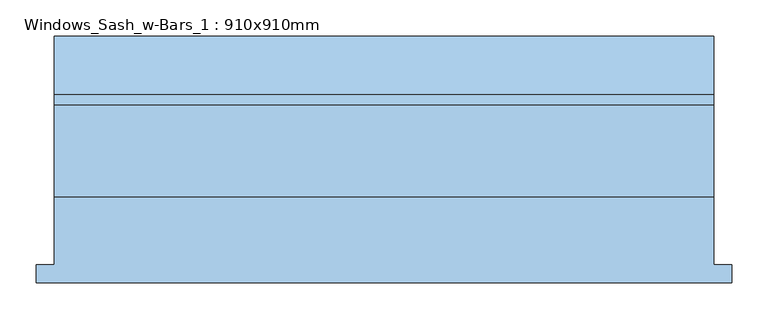
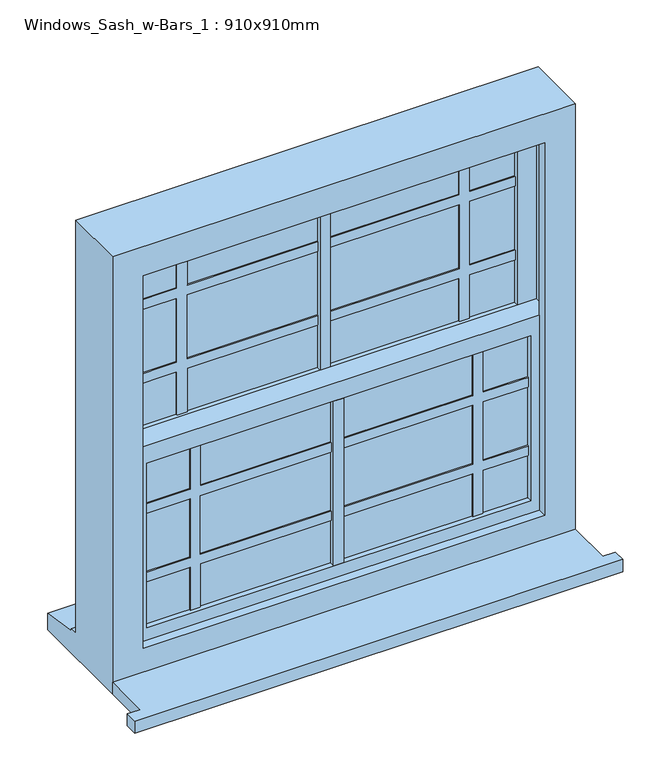
"""IFC4 building model written with IfcOpenShell, lengths in millimetres: window geometry, Windows_Sash_w-Bars_1 : 910x910mm."""

from ifc_helpers import new_model, si_unit, frame, origin, place, context, project, spatial, polyline, outline, extrude, faceted_brep, source, transform, mapped, element, save


def windows_sash_w_bars_1_910x910mm_b688f793(model_context):
    return source(origin(), model_context, "Body", "SolidModel", [
        extrude(outline(polyline([(-455.0, -101.6), (-455.0, -8.0), (455.0, -8.0), (455.0, -101.6), (480.0, -101.6), (480.0, -126.6), (-480.0, -126.6), (-480.0, -101.6), (-455.0, -101.6)])), frame((0.0, 0.0, 800.0), z_axis=(0.0, 0.0, 1.0), x_axis=(1.0, 0.0, 0.0)), (0.0, 0.0, 1.0), 25.0),
        faceted_brep([(377.9, 20.5, 1242.9), (377.9, 10.0, 1242.9), (-377.9, 10.0, 1242.9), (-377.9, 20.5, 1242.9), (387.9, 44.5, 1252.9), (387.9, 20.5, 1252.9), (-387.9, 20.5, 1252.9), (-387.9, 44.5, 1252.9), (377.9, 55.0, 1242.9), (377.9, 44.5, 1242.9), (-377.9, 44.5, 1242.9), (-377.9, 55.0, 1242.9), (415.0, 10.0, 1280.0), (415.0, 55.0, 1280.0), (-415.0, 55.0, 1280.0), (-415.0, 10.0, 1280.0), (-377.9, 10.0, 900.1), (-377.9, 20.5, 900.1), (-387.9, 20.5, 890.1), (-387.9, 44.5, 890.1), (-377.9, 44.5, 900.1), (-377.9, 55.0, 900.1), (-415.0, 55.0, 863.0), (-415.0, 10.0, 863.0), (377.9, 10.0, 900.1), (377.9, 20.5, 900.1), (387.9, 20.5, 890.1), (387.9, 44.5, 890.1), (377.9, 44.5, 900.1), (377.9, 55.0, 900.1), (415.0, 55.0, 863.0), (415.0, 10.0, 863.0)], [[[0, 1, 2, 3]], [[4, 5, 6, 7]], [[8, 9, 10, 11]], [[12, 13, 14, 15]], [[3, 2, 16, 17]], [[7, 6, 18, 19]], [[11, 10, 20, 21]], [[15, 14, 22, 23]], [[17, 16, 24, 25]], [[19, 18, 26, 27]], [[21, 20, 28, 29]], [[23, 22, 30, 31]], [[15, 23, 31, 12], [1, 24, 16, 2]], [[25, 24, 1, 0]], [[5, 26, 18, 6], [3, 17, 25, 0]], [[27, 26, 5, 4]], [[7, 19, 27, 4], [9, 28, 20, 10]], [[29, 28, 9, 8]], [[13, 30, 22, 14], [11, 21, 29, 8]], [[31, 30, 13, 12]]]),
        extrude(outline(polyline([(387.9, 20.5), (-387.9, 20.5), (-387.9, 44.5), (387.9, 44.5), (387.9, 20.5)])), frame((0.0, 0.0, 890.1), z_axis=(0.0, 0.0, 1.0), x_axis=(1.0, 0.0, 0.0)), (0.0, 0.0, 1.0), 362.8),
        extrude(outline(polyline([(387.9, 65.5), (-387.9, 65.5), (-387.9, 89.5), (387.9, 89.5), (387.9, 65.5)])), frame((0.0, 0.0, 1269.6), z_axis=(0.0, 0.0, 1.0), x_axis=(1.0, 0.0, 0.0)), (0.0, 0.0, 1.0), 373.3),
        extrude(outline(polyline([(1642.9, 267.9), (1542.9, 267.9), (1542.9, -267.9), (1642.9, -267.9), (1642.9, -287.9), (1542.9, -287.9), (1542.9, -387.9), (1522.9, -387.9), (1522.9, -287.9), (1389.6, -287.9), (1389.6, -387.9), (1369.6, -387.9), (1369.6, -287.9), (1269.6, -287.9), (1269.6, -267.9), (1369.6, -267.9), (1369.6, 267.9), (1269.6, 267.9), (1269.6, 287.9), (1369.6, 287.9), (1369.6, 387.9), (1389.6, 387.9), (1389.6, 287.9), (1522.9, 287.9), (1522.9, 387.9), (1542.9, 387.9), (1542.9, 287.9), (1642.9, 287.9), (1642.9, 267.9)]), holes=[polyline([(1522.9, -267.9), (1522.9, 267.9), (1389.6, 267.9), (1389.6, -267.9), (1522.9, -267.9)])]), frame((0.0, 62.5, 0.0), z_axis=(0.0, 1.0, 0.0), x_axis=(0.0, 0.0, 1.0)), (0.0, 0.0, 1.0), 30.0),
        extrude(outline(polyline([(1252.5, 267.9), (1152.5, 267.9), (1152.5, -267.9), (1252.5, -267.9), (1252.5, -287.9), (1152.5, -287.9), (1152.5, -387.9), (1132.5, -387.9), (1132.5, -287.9), (1010.1, -287.9), (1010.1, -387.9), (990.1, -387.9), (990.1, -287.9), (890.1, -287.9), (890.1, -267.9), (990.1, -267.9), (990.1, 267.9), (890.1, 267.9), (890.1, 287.9), (990.1, 287.9), (990.1, 387.9), (1010.1, 387.9), (1010.1, 287.9), (1132.5, 287.9), (1132.5, 387.9), (1152.5, 387.9), (1152.5, 287.9), (1252.5, 287.9), (1252.5, 267.9)]), holes=[polyline([(1132.5, -267.9), (1132.5, 267.9), (1010.1, 267.9), (1010.1, -267.9), (1132.5, -267.9)])]), frame((0.0, 17.5, 0.0), z_axis=(0.0, 1.0, 0.0), x_axis=(0.0, 0.0, 1.0)), (0.0, 0.0, 1.0), 30.0),
        faceted_brep([(-415.0, 55.0, 1670.0), (-415.0, 100.0, 1670.0), (-415.0, 100.0, 1192.5), (-415.0, 55.0, 1192.5), (-377.9, 65.5, 1632.9), (-377.9, 55.0, 1632.9), (-377.9, 55.0, 1279.6), (-377.9, 65.5, 1279.6), (-387.9, 89.5, 1642.9), (-387.9, 65.5, 1642.9), (-387.9, 65.5, 1269.6), (-387.9, 89.5, 1269.6), (-377.9, 100.0, 1632.9), (-377.9, 89.5, 1632.9), (-377.9, 89.5, 1279.6), (-377.9, 100.0, 1279.6), (-387.9, 55.0, 1242.5), (-387.9, 100.0, 1242.5), (387.9, 100.0, 1242.5), (387.9, 55.0, 1242.5), (377.9, 55.0, 1279.6), (377.9, 65.5, 1279.6), (387.9, 65.5, 1269.6), (387.9, 89.5, 1269.6), (377.9, 89.5, 1279.6), (377.9, 100.0, 1279.6), (415.0, 100.0, 1670.0), (415.0, 55.0, 1670.0), (415.0, 55.0, 1192.5), (415.0, 100.0, 1192.5), (377.9, 55.0, 1632.9), (377.9, 65.5, 1632.9), (387.9, 65.5, 1642.9), (387.9, 89.5, 1642.9), (377.9, 89.5, 1632.9), (377.9, 100.0, 1632.9), (-395.0, 55.0, 1192.5), (395.0, 55.0, 1192.5), (395.0, 100.0, 1192.5), (-395.0, 100.0, 1192.5)], [[[0, 1, 2, 3]], [[4, 5, 6, 7]], [[8, 9, 10, 11]], [[12, 13, 14, 15]], [[16, 17, 18, 19]], [[7, 6, 20, 21]], [[11, 10, 22, 23]], [[15, 14, 24, 25]], [[26, 27, 28, 29]], [[21, 20, 30, 31]], [[23, 22, 32, 33]], [[25, 24, 34, 35]], [[1, 0, 27, 26]], [[28, 27, 0, 3, 36, 16, 19, 37], [6, 5, 30, 20]], [[5, 4, 31, 30]], [[10, 9, 32, 22], [4, 7, 21, 31]], [[9, 8, 33, 32]], [[8, 11, 23, 33], [14, 13, 34, 24]], [[13, 12, 35, 34]], [[26, 29, 38, 18, 17, 39, 2, 1], [12, 15, 25, 35]], [[39, 36, 3, 2]], [[36, 39, 17, 16]], [[37, 38, 29, 28]], [[38, 37, 19, 18]]]),
        extrude(outline(polyline([(10.0, 100.0), (10.0, 55.0), (-10.0, 55.0), (-10.0, 100.0), (10.0, 100.0)])), frame((0.0, 0.0, 1279.6), z_axis=(0.0, 0.0, 1.0), x_axis=(1.0, 0.0, 0.0)), (0.0, 0.0, 1.0), 353.3),
        extrude(outline(polyline([(10.0, 55.0), (10.0, 10.0), (-10.0, 10.0), (-10.0, 55.0), (10.0, 55.0)])), frame((0.0, 0.0, 900.1), z_axis=(0.0, 0.0, 1.0), x_axis=(1.0, 0.0, 0.0)), (0.0, 0.0, 1.0), 342.4),
        faceted_brep([(455.0, -8.0, 1710.0), (-455.0, -8.0, 1710.0), (-455.0, -8.0, 800.0), (455.0, -8.0, 800.0), (395.0, -8.0, 1650.0), (395.0, -8.0, 875.0), (-395.0, -8.0, 875.0), (-395.0, -8.0, 1650.0), (395.0, 10.0, 1650.0), (395.0, 10.0, 875.0), (-415.0, 10.0, 1670.0), (415.0, 10.0, 1670.0), (415.0, 10.0, 863.0), (-415.0, 10.0, 863.0), (-395.0, 10.0, 1650.0), (-395.0, 10.0, 875.0), (415.0, 100.0, 1670.0), (415.0, 100.0, 863.0), (-415.0, 100.0, 1670.0), (-415.0, 100.0, 863.0), (-395.0, 100.0, 863.0), (-395.0, 100.0, 1650.0), (395.0, 100.0, 1650.0), (395.0, 100.0, 863.0), (395.0, 118.0, 1650.0), (395.0, 118.0, 863.0), (455.0, 118.0, 851.0), (-455.0, 118.0, 851.0), (-455.0, 118.0, 1710.0), (455.0, 118.0, 1710.0), (-395.0, 118.0, 1650.0), (-395.0, 118.0, 863.0), (455.0, 213.5, 800.0), (455.0, 213.5, 833.8), (455.0, 133.0, 846.7), (455.0, 133.0, 850.4), (-455.0, 133.0, 850.4), (-455.0, 133.0, 846.7), (-455.0, 213.5, 833.8), (-455.0, 213.5, 800.0)], [[[0, 1, 2, 3], [4, 5, 6, 7]], [[4, 8, 9, 5]], [[10, 11, 12, 13], [8, 14, 15, 9]], [[12, 11, 16, 17]], [[17, 16, 18, 19, 20, 21, 22, 23]], [[23, 22, 24, 25]], [[26, 27, 28, 29], [25, 24, 30, 31]], [[26, 29, 0, 3, 32, 33, 34, 35]], [[4, 7, 14, 8]], [[11, 10, 18, 16]], [[22, 21, 30, 24]], [[1, 0, 29, 28]], [[14, 7, 6, 15]], [[19, 18, 10, 13]], [[21, 20, 31, 30]], [[28, 27, 36, 37, 38, 39, 2, 1]], [[9, 15, 6, 5]], [[13, 12, 17, 23, 25, 31, 20, 19]], [[36, 27, 26, 35]], [[37, 36, 35, 34]], [[38, 37, 34, 33]], [[39, 38, 33, 32]], [[2, 39, 32, 3]]]),
    ])


if __name__ == "__main__":
    model = new_model("IFC4")
    model_context = context("Model", 3, world=origin())
    ifc_project = project(units=[si_unit("LENGTHUNIT", "METRE", prefix="MILLI")], contexts=[model_context])
    site = spatial("IfcSite", under=ifc_project)
    building = spatial("IfcBuilding", under=site)
    placement = place(None, origin())
    windows_sash_w_bars_1_910x910mm_shape = windows_sash_w_bars_1_910x910mm_b688f793(model_context)
    element("IfcWindow", 1, ObjectType="Windows_Sash_w-Bars_1 : 910x910mm", at=placement, inside=building, context=model_context, shape_type="MappedRepresentation", body=[
        mapped(windows_sash_w_bars_1_910x910mm_shape, transform((0.0, 0.0, 0.0), x_axis=(1.0, 0.0, 0.0), y_axis=(0.0, 1.0, 0.0), z_axis=(0.0, 0.0, 1.0))),
    ])
    save(model, "model.ifc")

# Revit data of these elements
# Type "Windows_Sash_w-Bars_1 : 910x910mm"
#   Type Mark = "24"
#   Construction Type Id = "GSP4R"
#   Analytic Construction = "1/8 in Pilkington single glazing"
#   Wrap Layers (Int) from Ext = 0' - 6.98819"
#   Wrap Layers (Ext) from Ext = 0' - 4.03543"
#   Window Board Projection = 0' - 0.98425"
#   Window Board Extension = 0' - 0.98425"
#   Visual Light Transmittance = 0.9
#   Solar Heat Gain Coefficient = 0.78
#   Rough Width = 2' - 11.82677"
#   Rough Height = 2' - 11.82677"
#   Height = 2' - 11.82677"
#   Heat Transfer Coefficient (U) = 0.6496 BTU/(h·ft²·°F)
#   Glazing Thickness = 0' - 0.94488"
#   Glazing Bar Offset = 0' - 3.93701"
#   Frame Depth = 0' - 3.54331"
#   FrameOffset - External = 0' - 1.9685"
#   Default Sill Height = 2' - 7.49606"
#   Width = 2' - 11.82677"
#   Glazing Bar Thickness = 0' - 0.7874"
#   Cavity Closer Width = 0' - 1.9685"
#   Cavity Closer Offset from Ext = 0' - 4.03543"
#   Cavity Closer Depth = 0' - 3.34646"
#   Vis - Vert Bar Top = yes
#   Vis - Vert Bar Bttm = yes
#   Vis - Glazing Bars Top = yes
#   Vis - Glazing Bars Bttm = yes
#   Vis - Cavity Closers = yes
#   Define Thermal Properties by = 1
#   Material Trim = Window Frame
#   Material Frame = Window Frame
#   Material Glazing Bars = Window Frame
#   Material Glass = Glass
#   Wall Closure = (empty or 0)
# Element 1 (IfcWindow, "Windows_Sash_w-Bars_1 : 910x910mm")
#   Materials on its faces: "Window Frame", "Glass"
# Materials
#   "Window Frame": colour RGB 249 249 249, transparency 0
#   "Glass": class "Glass", colour RGB 0 128 192, transparency 0.75, Description = "Soda Lime Glass", Cost = 0
